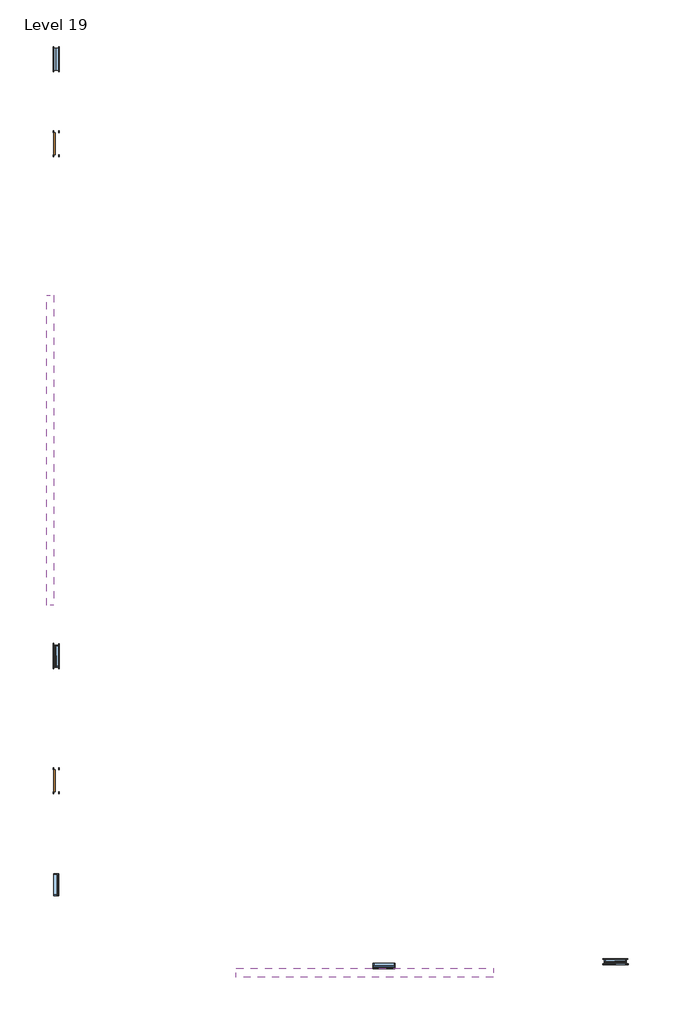
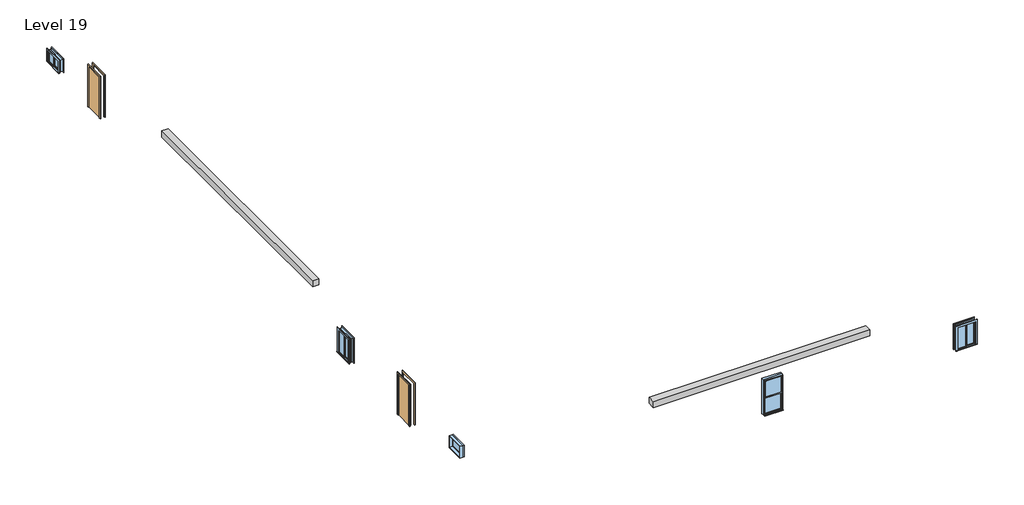
# One storey: 5 windows, 2 doors, 2 proxies.
"""IFC4 building model written with IfcOpenShell, lengths in millimetres."""

from ifc_helpers import new_model, si_unit, origin, place, context, project, spatial, transform, mapped, element, save
from components import generic_models_13_generic_models_13_7be0e28e, generic_models_2_generic_models_2_383bbf5d, door_54dd4da4, window_f274a882, window_57c3ee1c, window_a4355bb3, window_54100e87

model = new_model("IFC4")

# Units and contexts
model_context = context("Model", 3, world=origin())
ifc_project = project(units=[si_unit("LENGTHUNIT", "METRE", prefix="MILLI")], contexts=[model_context])

# Site, building, storey
site = spatial("IfcSite", under=ifc_project)
building = spatial("IfcBuilding", under=site)
storey = spatial("IfcBuildingStorey", under=building, Name="Level 19", Elevation=29870.4)

# Proxies
placement = place(None, origin())
generic_models_13_generic_models_13_shape = generic_models_13_generic_models_13_7be0e28e(model_context)
element("IfcBuildingElementProxy", 1, Name="Generic Models 13 : Generic Models 13", ObjectType="Generic Models 13 : Generic Models 13", at=placement, inside=storey, context=model_context, shape_type="MappedRepresentation", body=[
    mapped(generic_models_13_generic_models_13_shape, transform((0.0, 0.0, 0.0), x_axis=(1.0, 0.0, 0.0), y_axis=(0.0, 1.0, 0.0), z_axis=(0.0, 0.0, 1.0))),
])
generic_models_2_generic_models_2_shape = generic_models_2_generic_models_2_383bbf5d(model_context)
element("IfcBuildingElementProxy", 2, Name="Generic Models 2 : Generic Models 2", ObjectType="Generic Models 2 : Generic Models 2", at=placement, inside=storey, context=model_context, shape_type="MappedRepresentation", body=[
    mapped(generic_models_2_generic_models_2_shape, transform((0.0, 0.0, 0.0), x_axis=(1.0, 0.0, 0.0), y_axis=(0.0, 1.0, 0.0), z_axis=(0.0, 0.0, 1.0))),
])

# Doors
door_shape = door_54dd4da4(model_context)
element("IfcDoor", 3, ObjectType="Single-Flush : 36\" x 84\"", at=placement, inside=storey, context=model_context, shape_type="MappedRepresentation", body=[
    mapped(door_shape, transform((-15175.038074, 13190.2014639, 29870.4), x_axis=(0.0, 1.0, 0.0), y_axis=(-1.0, 0.0, 0.0), z_axis=(0.0, 0.0, 1.0))),
])
element("IfcDoor", 4, ObjectType="Single-Flush : 36\" x 84\"", at=placement, inside=storey, context=model_context, shape_type="MappedRepresentation", body=[
    mapped(door_shape, transform((-15175.038074, -13242.9915889, 29870.4), x_axis=(0.0, 1.0, 0.0), y_axis=(-1.0, 0.0, 0.0), z_axis=(0.0, 0.0, 1.0))),
])

# Windows
window_shape = window_f274a882(model_context)
element("IfcWindow", 5, ObjectType="Double Hung : 36\" x 72\"", at=placement, inside=storey, context=model_context, shape_type="MappedRepresentation", body=[
    mapped(window_shape, transform((-1560.638074, -20921.9985361, 29870.4), x_axis=(-1.0, 0.0, 0.0), y_axis=(0.0, -1.0, 0.0), z_axis=(0.0, 0.0, 1.0))),
])
window_2_shape = window_57c3ee1c(model_context)
element("IfcWindow", 6, ObjectType="Fixed : 36\" x 24\"", at=placement, inside=storey, context=model_context, shape_type="MappedRepresentation", body=[
    mapped(window_2_shape, transform((-15175.038074, -17587.3213044, 29870.4), x_axis=(0.0, -1.0, 0.0), y_axis=(1.0, 0.0, 0.0), z_axis=(0.0, 0.0, 1.0))),
])
window_3_shape = window_a4355bb3(model_context)
element("IfcWindow", 7, ObjectType="Slider with Trim : 36\" x 24\"", at=placement, inside=storey, context=model_context, shape_type="MappedRepresentation", body=[
    mapped(window_3_shape, transform((-15175.038074, 16695.4014639, 29194.6975007), x_axis=(0.0, 1.0, 0.0), y_axis=(-1.0, 0.0, 0.0), z_axis=(0.0, 0.0, 1.0))),
])
window_4_shape = window_54100e87(model_context)
element("IfcWindow", 8, ObjectType="Slider with Trim : 36\" x 48\"", at=placement, inside=storey, context=model_context, shape_type="MappedRepresentation", body=[
    mapped(window_4_shape, transform((8040.561926, -20744.1985361, 29193.7828035), x_axis=(-1.0, 0.0, 0.0), y_axis=(0.0, -1.0, 0.0), z_axis=(0.0, 0.0, 1.0))),
])
element("IfcWindow", 9, ObjectType="Slider with Trim : 36\" x 48\"", at=placement, inside=storey, context=model_context, shape_type="MappedRepresentation", body=[
    mapped(window_4_shape, transform((-15175.038074, -8075.0213044, 29077.9058376), x_axis=(0.0, 1.0, 0.0), y_axis=(-1.0, 0.0, 0.0), z_axis=(0.0, 0.0, 1.0))),
])

save(model, "model.ifc")

# Revit data of these elements
# Type "Single-Flush : 36\" x 84\""
#   Type Mark = "1"
#   Construction Type Id = "MDOOR"
#   Assembly Code = "C1020"
#   Analytic Construction = "Metal"
#   Thickness = 0' - 2"
#   Heat Transfer Coefficient (U) = 0.651978 BTU/(h·ft²·°F)
#   Height = 7' - 0"
#   Trim Projection Ext = 0' - 1"
#   Trim Projection Int = 0' - 1"
#   Trim Width = 0' - 3"
#   Width = 3' - 0"
#   Define Thermal Properties by = 1
#   Door Material = Door - Panel
#   Frame Material = Door - Frame
#   Visual Light Transmittance = 0
#   Solar Heat Gain Coefficient = 0
#   Function = (empty or 0)
#   Wall Closure = (empty or 0)
# Type "Double Hung : 36\" x 72\""
#   Type Mark = "18"
#   Construction Type Id = "GSP4R"
#   Assembly Code = "B2020100"
#   Analytic Construction = "1/8 in Pilkington single glazing"
#   Visual Light Transmittance = 0.9
#   Solar Heat Gain Coefficient = 0.78
#   Heat Transfer Coefficient (U) = 0.6496 BTU/(h·ft²·°F)
#   Height = 6' - 0"
#   Default Sill Height = 1' - 0"
#   Width = 3' - 0"
#   Window Inset = 0' - 0 3/4"
#   Define Thermal Properties by = 1
#   Glass Pane Material = Glass
#   Sash Material = Sash
#   Description = (empty or 0)
#   Wall Closure = (empty or 0)
# Type "Fixed : 36\" x 24\""
#   Type Mark = "8"
#   Construction Type Id = "GSP4R"
#   Assembly Code = "B2020100"
#   Analytic Construction = "1/8 in Pilkington single glazing"
#   Visual Light Transmittance = 0.9
#   Solar Heat Gain Coefficient = 0.78
#   Heat Transfer Coefficient (U) = 0.6496 BTU/(h·ft²·°F)
#   Height = 2' - 0"
#   Default Sill Height = 3' - 0"
#   Width = 3' - 0"
#   Window Inset = 0' - 0 3/4"
#   Define Thermal Properties by = 1
#   Glass Pane Material = Glass
#   Sash Material = Sash
#   Wall Closure = (empty or 0)
# Type "Slider with Trim : 36\" x 24\""
#   Type Mark = "23"
#   Construction Type Id = "GSP4R"
#   Assembly Code = "B2020100"
#   Analytic Construction = "1/8 in Pilkington single glazing"
#   Visual Light Transmittance = 0.9
#   Solar Heat Gain Coefficient = 0.78
#   Heat Transfer Coefficient (U) = 0.6496 BTU/(h·ft²·°F)
#   Height = 2' - 0"
#   Default Sill Height = 3' - 0"
#   Trim Projection - Ext. = 0' - 0 3/4"
#   Trim Projection - Int. = 0' - 0 3/4"
#   Trim Width - Exterior = 0' - 3 1/2"
#   Trim Width - Interior = 0' - 3 1/2"
#   Width = 3' - 0"
#   Window Inset = 0' - 0 3/4"
#   Define Thermal Properties by = 1
#   Glass Pane Material = Glass
#   Sash Material = Sash
#   Trim Exterior Material = Trim
#   Trim Interior Material = Trim
#   Wall Closure = (empty or 0)
# Type "Slider with Trim : 36\" x 48\""
#   Type Mark = "22"
#   Construction Type Id = "GSP4R"
#   Assembly Code = "B2020100"
#   Analytic Construction = "1/8 in Pilkington single glazing"
#   Visual Light Transmittance = 0.9
#   Solar Heat Gain Coefficient = 0.78
#   Heat Transfer Coefficient (U) = 0.6496 BTU/(h·ft²·°F)
#   Height = 4' - 0"
#   Default Sill Height = 3' - 0"
#   Trim Projection - Ext. = 0' - 0 3/4"
#   Trim Projection - Int. = 0' - 0 3/4"
#   Trim Width - Exterior = 0' - 3 1/2"
#   Trim Width - Interior = 0' - 3 1/2"
#   Width = 3' - 0"
#   Window Inset = 0' - 0 3/4"
#   Define Thermal Properties by = 1
#   Glass Pane Material = Glass
#   Sash Material = Sash
#   Trim Exterior Material = Trim
#   Trim Interior Material = Trim
#   Wall Closure = (empty or 0)
# Element 1 (IfcBuildingElementProxy, "Generic Models 13 : Generic Models 13")
#   Phase Created = New Construction
# Element 2 (IfcBuildingElementProxy, "Generic Models 2 : Generic Models 2")
#   Phase Created = New Construction
# Elements 3, 4 (IfcDoor, "Single-Flush : 36\" x 84\"")
#   Phase Created = New Construction
#   Materials on its faces: "Door - Frame", "Door - Panel"
# Element 5 (IfcWindow, "Double Hung : 36\" x 72\"")
#   Mark = "3"
#   Phase Created = New Construction
#   Materials on its faces: "Sash", "Glass"
# Element 6 (IfcWindow, "Fixed : 36\" x 24\"")
#   Mark = "69"
#   Phase Created = New Construction
#   Materials on its faces: "Sash", "Glass"
# Element 7 (IfcWindow, "Slider with Trim : 36\" x 24\"")
#   Mark = "58"
#   Phase Created = New Construction
#   Materials on its faces: "Sash", "Trim", "Glass"
# Element 8 (IfcWindow, "Slider with Trim : 36\" x 48\"")
#   Mark = "25"
#   Phase Created = New Construction
#   Materials on its faces: "Sash", "Trim", "Glass"
# Element 9 (IfcWindow, "Slider with Trim : 36\" x 48\"")
#   Mark = "36"
#   Phase Created = New Construction
#   Materials on its faces: "Sash", "Trim", "Glass"
# Materials
#   "Door - Panel": class "Wood", colour RGB 210 159 95, transparency 0
#   "Door - Frame": colour RGB 118 70 51, transparency 0
#   "Glass": class "Glass", colour RGB 0 128 192, transparency 0.75, Description = "Soda Lime Glass", Cost = 0
#   "Sash": class "Wood", colour RGB 224 178 126, transparency 0
#   "Trim": class "Wood", colour RGB 224 178 126, transparency 0
